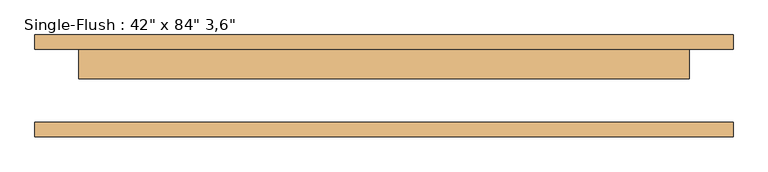
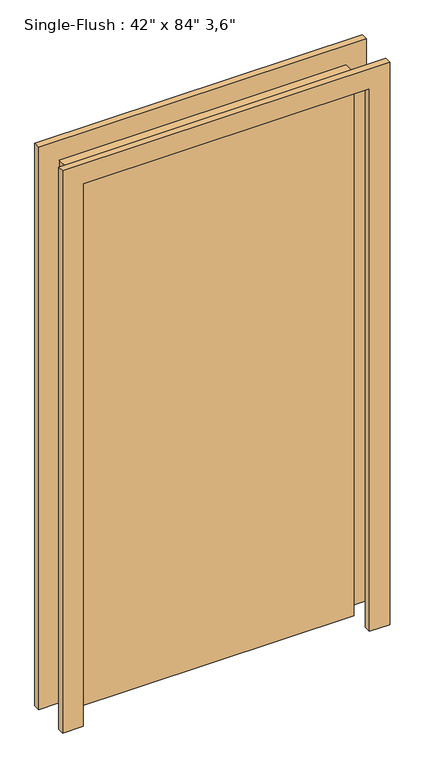
"""IFC4 building model written with IfcOpenShell, lengths in millimetres: door geometry."""

from ifc_helpers import new_model, si_unit, frame, origin, origin_with_axes, place, context, project, spatial, polyline, outline, extrude, source, transform, mapped, element, save


def door_4f94b823(model_context):
    return source(origin(), model_context, "Body", "SweptSolid", [
        extrude(outline(polyline([(2209.8, -609.6), (0.0, -609.6), (0.0, -533.4), (2133.6, -533.4), (2133.6, 533.4), (0.0, 533.4), (0.0, 609.6), (2209.8, 609.6), (2209.8, -609.6)])), frame((0.0, 63.5, 0.0), z_axis=(0.0, 1.0, 0.0), x_axis=(0.0, 0.0, 1.0)), (0.0, 0.0, 1.0), 25.4),
        extrude(outline(polyline([(2209.8, 609.6), (2209.8, -609.6), (0.0, -609.6), (0.0, -533.4), (2133.6, -533.4), (2133.6, 533.4), (0.0, 533.4), (0.0, 609.6), (2209.8, 609.6)])), frame((0.0, -88.9, 0.0), z_axis=(0.0, 1.0, 0.0), x_axis=(0.0, 0.0, 1.0)), (0.0, 0.0, 1.0), 25.4),
        extrude(outline(polyline([(533.4, 12.7), (-533.4, 12.7), (-533.4, 63.5), (533.4, 63.5), (533.4, 12.7)])), origin_with_axes(), (0.0, 0.0, 1.0), 2133.6),
    ])


if __name__ == "__main__":
    model = new_model("IFC4")
    model_context = context("Model", 3, world=origin())
    ifc_project = project(units=[si_unit("LENGTHUNIT", "METRE", prefix="MILLI")], contexts=[model_context])
    site = spatial("IfcSite", under=ifc_project)
    building = spatial("IfcBuilding", under=site)
    placement = place(None, origin())
    door_shape = door_4f94b823(model_context)
    element("IfcDoor", 1, ObjectType="Single-Flush : 42\" x 84\" 3,6\"", at=placement, inside=building, context=model_context, shape_type="MappedRepresentation", body=[
        mapped(door_shape, transform((0.0, 0.0, 0.0), x_axis=(1.0, 0.0, 0.0), y_axis=(0.0, 1.0, 0.0), z_axis=(0.0, 0.0, 1.0))),
    ])
    save(model, "model.ifc")

# Revit data of these elements
# Type "Single-Flush : 42\" x 84\" 3,6\""
#   Type Mark = "8"
#   Assembly Code = "C1020"
#   Thickness = 0' - 2"
#   Height = 7' - 0"
#   Trim Projection Ext = 0' - 1"
#   Trim Projection Int = 0' - 1"
#   Trim Width = 0' - 3"
#   Width = 3' - 6"
#   Door Material = Door - Panel
#   Frame Material = Door - Frame
#   Function = (empty or 0)
#   Wall Closure = (empty or 0)
# Element 1 (IfcDoor, "Single-Flush : 42\" x 84\" 3,6\"")
#   Materials on its faces: "Door - Frame", "Door - Panel"
# Materials
#   "Door - Panel": class "Wood", colour RGB 114 82 51, transparency 0
#   "Door - Frame": colour RGB 153 76 43, transparency 0
